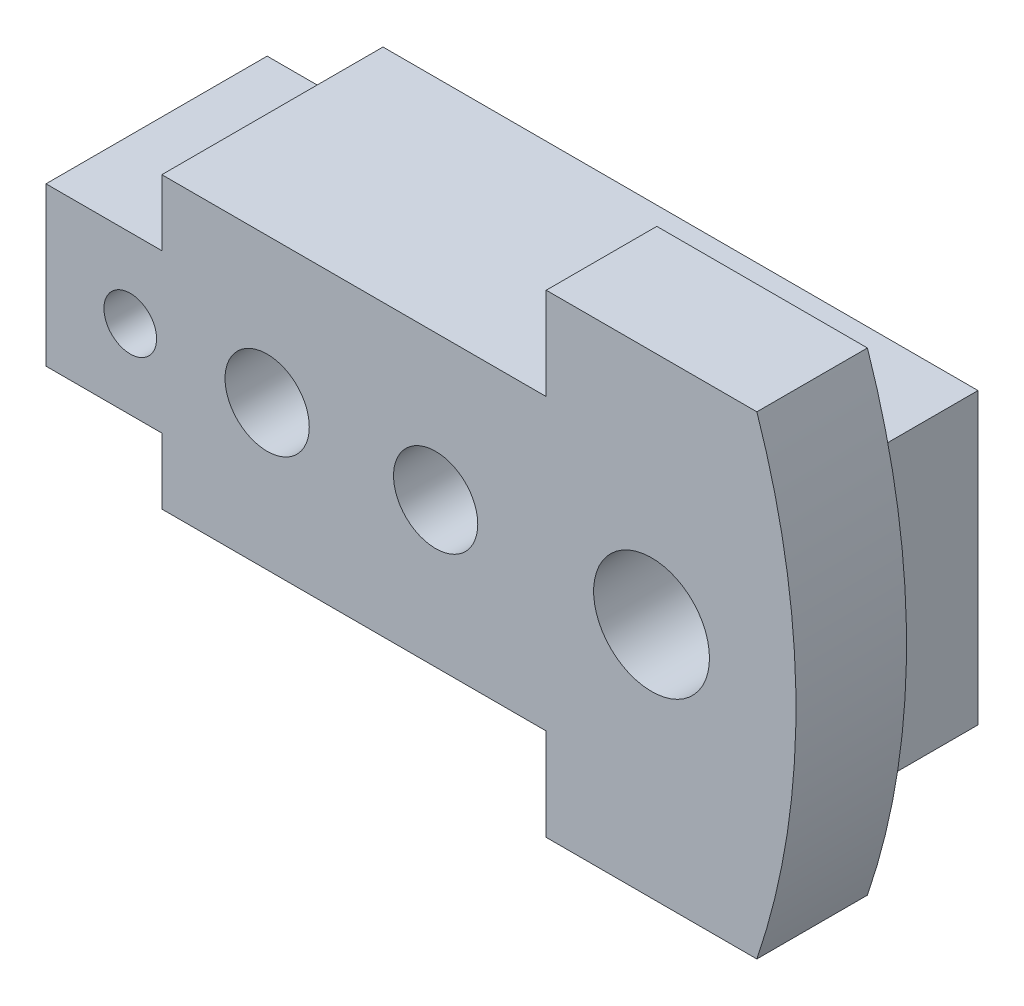
ISO-10303-21;
HEADER;
FILE_DESCRIPTION(('STEP AP214'),'2;1');
FILE_NAME('part.step','',(''),(''),'','','');
FILE_SCHEMA(('AUTOMOTIVE_DESIGN { 1 0 10303 214 1 1 1 1 }'));
ENDSEC;
DATA;
#1=APPLICATION_CONTEXT('core data for automotive mechanical design processes');
#2=APPLICATION_PROTOCOL_DEFINITION('international standard','automotive_design',2000,#1);
#3=PRODUCT_CONTEXT('',#1,'mechanical');
#4=PRODUCT('Part','Part','',(#3));
#5=PRODUCT_RELATED_PRODUCT_CATEGORY('part','',(#4));
#6=PRODUCT_DEFINITION_FORMATION('','',#4);
#7=PRODUCT_DEFINITION_CONTEXT('part definition',#1,'design');
#8=PRODUCT_DEFINITION('design','',#6,#7);
#9=PRODUCT_DEFINITION_SHAPE('','',#8);
#10=(LENGTH_UNIT() NAMED_UNIT(*) SI_UNIT(.MILLI.,.METRE.));
#11=(NAMED_UNIT(*) PLANE_ANGLE_UNIT() SI_UNIT($,.RADIAN.));
#12=(NAMED_UNIT(*) SI_UNIT($,.STERADIAN.) SOLID_ANGLE_UNIT());
#13=UNCERTAINTY_MEASURE_WITH_UNIT(LENGTH_MEASURE(1.E-05),#10,'distance_accuracy_value','');
#14=(GEOMETRIC_REPRESENTATION_CONTEXT(3) GLOBAL_UNCERTAINTY_ASSIGNED_CONTEXT((#13)) GLOBAL_UNIT_ASSIGNED_CONTEXT((#10,
#11,#12)) REPRESENTATION_CONTEXT('',''));
#15=CARTESIAN_POINT('',(0.,0.,0.));
#16=DIRECTION('',(0.,0.,1.));
#17=DIRECTION('',(1.,0.,0.));
#18=AXIS2_PLACEMENT_3D('',#15,#16,#17);
#19=CARTESIAN_POINT('',(0.,0.,0.));
#20=DIRECTION('',(0.,0.,1.));
#21=DIRECTION('',(1.,0.,0.));
#22=AXIS2_PLACEMENT_3D('',#19,#20,#21);
#23=PLANE('',#22);
#24=DIRECTION('',(0.,-1.,0.));
#25=VECTOR('',#24,1.);
#26=CARTESIAN_POINT('',(18.,0.,0.));
#27=LINE('',#26,#25);
#28=CARTESIAN_POINT('',(18.,72.5,0.));
#29=VERTEX_POINT('',#28);
#30=CARTESIAN_POINT('',(18.,60.,0.));
#31=VERTEX_POINT('',#30);
#32=EDGE_CURVE('E70',#29,#31,#27,.T.);
#33=ORIENTED_EDGE('',*,*,#32,.F.);
#34=DIRECTION('',(1.,0.,0.));
#35=VECTOR('',#34,1.);
#36=CARTESIAN_POINT('',(91.,72.5,0.));
#37=LINE('',#36,#35);
#38=CARTESIAN_POINT('',(131.,72.5,0.));
#39=VERTEX_POINT('',#38);
#40=EDGE_CURVE('E153',#29,#39,#37,.T.);
#41=ORIENTED_EDGE('',*,*,#40,.T.);
#42=DIRECTION('',(0.,1.,0.));
#43=VECTOR('',#42,1.);
#44=CARTESIAN_POINT('',(131.,90.,0.));
#45=LINE('',#44,#43);
#46=CARTESIAN_POINT('',(131.,17.5,0.));
#47=VERTEX_POINT('',#46);
#48=EDGE_CURVE('E188',#47,#39,#45,.T.);
#49=ORIENTED_EDGE('',*,*,#48,.F.);
#50=DIRECTION('',(1.,0.,0.));
#51=VECTOR('',#50,1.);
#52=CARTESIAN_POINT('',(91.,17.5,0.));
#53=LINE('',#52,#51);
#54=CARTESIAN_POINT('',(18.,17.5,0.));
#55=VERTEX_POINT('',#54);
#56=EDGE_CURVE('E234',#55,#47,#53,.T.);
#57=ORIENTED_EDGE('',*,*,#56,.F.);
#58=DIRECTION('',(0.,-1.,0.));
#59=VECTOR('',#58,1.);
#60=CARTESIAN_POINT('',(18.,0.,0.));
#61=LINE('',#60,#59);
#62=CARTESIAN_POINT('',(18.,30.,0.));
#63=VERTEX_POINT('',#62);
#64=EDGE_CURVE('E195',#63,#55,#61,.T.);
#65=ORIENTED_EDGE('',*,*,#64,.F.);
#66=DIRECTION('',(-1.,0.,0.));
#67=VECTOR('',#66,1.);
#68=CARTESIAN_POINT('',(0.,30.,0.));
#69=LINE('',#68,#67);
#70=CARTESIAN_POINT('',(-3.99999999999999,30.,0.));
#71=VERTEX_POINT('',#70);
#72=EDGE_CURVE('E204',#63,#71,#69,.T.);
#73=ORIENTED_EDGE('',*,*,#72,.T.);
#74=DIRECTION('',(0.,-1.,0.));
#75=VECTOR('',#74,1.);
#76=CARTESIAN_POINT('',(-3.99999999999999,90.,0.));
#77=LINE('',#76,#75);
#78=CARTESIAN_POINT('',(-3.99999999999999,60.,0.));
#79=VERTEX_POINT('',#78);
#80=EDGE_CURVE('E11',#79,#71,#77,.T.);
#81=ORIENTED_EDGE('',*,*,#80,.F.);
#82=DIRECTION('',(1.,0.,0.));
#83=VECTOR('',#82,1.);
#84=CARTESIAN_POINT('',(0.,60.,0.));
#85=LINE('',#84,#83);
#86=EDGE_CURVE('E192',#79,#31,#85,.T.);
#87=ORIENTED_EDGE('',*,*,#86,.T.);
#88=EDGE_LOOP('',(#33,#41,#49,#57,#65,#73,#81,#87));
#89=FACE_BOUND('',#88,.T.);
#90=ADVANCED_FACE('F44',(#89),#23,.F.);
#91=CARTESIAN_POINT('',(131.,0.,0.));
#92=DIRECTION('',(-1.,0.,0.));
#93=DIRECTION('',(0.,0.,1.));
#94=AXIS2_PLACEMENT_3D('',#91,#92,#93);
#95=PLANE('',#94);
#96=DIRECTION('',(0.,0.,1.));
#97=VECTOR('',#96,1.);
#98=CARTESIAN_POINT('',(131.,72.5,0.));
#99=LINE('',#98,#97);
#100=CARTESIAN_POINT('',(131.,72.5,21.));
#101=VERTEX_POINT('',#100);
#102=EDGE_CURVE('E232',#39,#101,#99,.T.);
#103=ORIENTED_EDGE('',*,*,#102,.T.);
#104=DIRECTION('',(0.,-1.,0.));
#105=VECTOR('',#104,1.);
#106=CARTESIAN_POINT('',(131.,90.,21.));
#107=LINE('',#106,#105);
#108=CARTESIAN_POINT('',(131.,17.5,21.));
#109=VERTEX_POINT('',#108);
#110=EDGE_CURVE('E173',#101,#109,#107,.T.);
#111=ORIENTED_EDGE('',*,*,#110,.T.);
#112=DIRECTION('',(0.,0.,-1.));
#113=VECTOR('',#112,1.);
#114=CARTESIAN_POINT('',(131.,17.5,0.));
#115=LINE('',#114,#113);
#116=EDGE_CURVE('E58',#109,#47,#115,.T.);
#117=ORIENTED_EDGE('',*,*,#116,.T.);
#118=ORIENTED_EDGE('',*,*,#48,.T.);
#119=EDGE_LOOP('',(#103,#111,#117,#118));
#120=FACE_BOUND('',#119,.T.);
#121=ADVANCED_FACE('F338',(#120),#95,.F.);
#122=CARTESIAN_POINT('',(0.,0.,63.));
#123=DIRECTION('',(0.,1.,0.));
#124=DIRECTION('',(0.,0.,1.));
#125=AXIS2_PLACEMENT_3D('',#122,#123,#124);
#126=PLANE('',#125);
#127=DIRECTION('',(1.,0.,0.));
#128=VECTOR('',#127,1.);
#129=CARTESIAN_POINT('',(91.,0.,42.));
#130=LINE('',#129,#128);
#131=CARTESIAN_POINT('',(91.,0.,42.));
#132=VERTEX_POINT('',#131);
#133=CARTESIAN_POINT('',(131.,0.,42.));
#134=VERTEX_POINT('',#133);
#135=EDGE_CURVE('E182',#132,#134,#130,.T.);
#136=ORIENTED_EDGE('',*,*,#135,.F.);
#137=DIRECTION('',(0.,0.,1.));
#138=VECTOR('',#137,1.);
#139=CARTESIAN_POINT('',(91.,0.,42.));
#140=LINE('',#139,#138);
#141=CARTESIAN_POINT('',(91.,0.,21.));
#142=VERTEX_POINT('',#141);
#143=EDGE_CURVE('E239',#142,#132,#140,.T.);
#144=ORIENTED_EDGE('',*,*,#143,.F.);
#145=DIRECTION('',(1.,0.,0.));
#146=VECTOR('',#145,1.);
#147=CARTESIAN_POINT('',(91.,0.,21.));
#148=LINE('',#147,#146);
#149=CARTESIAN_POINT('',(131.,0.,21.));
#150=VERTEX_POINT('',#149);
#151=EDGE_CURVE('E236',#142,#150,#148,.T.);
#152=ORIENTED_EDGE('',*,*,#151,.T.);
#153=DIRECTION('',(0.,0.,-1.));
#154=VECTOR('',#153,1.);
#155=CARTESIAN_POINT('',(131.,0.,0.));
#156=LINE('',#155,#154);
#157=EDGE_CURVE('E190',#134,#150,#156,.T.);
#158=ORIENTED_EDGE('',*,*,#157,.F.);
#159=EDGE_LOOP('',(#136,#144,#152,#158));
#160=FACE_BOUND('',#159,.T.);
#161=ADVANCED_FACE('F50',(#160),#126,.F.);
#162=CARTESIAN_POINT('',(22.,90.,63.));
#163=DIRECTION('',(0.,-1.,0.));
#164=DIRECTION('',(0.,0.,-1.));
#165=AXIS2_PLACEMENT_3D('',#162,#163,#164);
#166=PLANE('',#165);
#167=DIRECTION('',(1.,0.,0.));
#168=VECTOR('',#167,1.);
#169=CARTESIAN_POINT('',(91.,90.,21.));
#170=LINE('',#169,#168);
#171=CARTESIAN_POINT('',(91.,90.,21.));
#172=VERTEX_POINT('',#171);
#173=CARTESIAN_POINT('',(131.,90.,21.));
#174=VERTEX_POINT('',#173);
#175=EDGE_CURVE('E260',#172,#174,#170,.T.);
#176=ORIENTED_EDGE('',*,*,#175,.F.);
#177=DIRECTION('',(0.,0.,-1.));
#178=VECTOR('',#177,1.);
#179=CARTESIAN_POINT('',(91.,90.,0.));
#180=LINE('',#179,#178);
#181=CARTESIAN_POINT('',(91.,90.,42.));
#182=VERTEX_POINT('',#181);
#183=EDGE_CURVE('E156',#182,#172,#180,.T.);
#184=ORIENTED_EDGE('',*,*,#183,.F.);
#185=DIRECTION('',(-1.,0.,0.));
#186=VECTOR('',#185,1.);
#187=CARTESIAN_POINT('',(91.,90.,42.));
#188=LINE('',#187,#186);
#189=CARTESIAN_POINT('',(131.,90.,42.));
#190=VERTEX_POINT('',#189);
#191=EDGE_CURVE('E184',#190,#182,#188,.T.);
#192=ORIENTED_EDGE('',*,*,#191,.F.);
#193=DIRECTION('',(0.,0.,1.));
#194=VECTOR('',#193,1.);
#195=CARTESIAN_POINT('',(131.,90.,21.));
#196=LINE('',#195,#194);
#197=EDGE_CURVE('E166',#174,#190,#196,.T.);
#198=ORIENTED_EDGE('',*,*,#197,.F.);
#199=EDGE_LOOP('',(#176,#184,#192,#198));
#200=FACE_BOUND('',#199,.T.);
#201=ADVANCED_FACE('F281',(#200),#166,.F.);
#202=CARTESIAN_POINT('',(-3.99999999999999,90.,63.));
#203=DIRECTION('',(1.,0.,0.));
#204=DIRECTION('',(0.,0.,-1.));
#205=AXIS2_PLACEMENT_3D('',#202,#203,#204);
#206=PLANE('',#205);
#207=DIRECTION('',(0.,0.,1.));
#208=VECTOR('',#207,1.);
#209=CARTESIAN_POINT('',(-3.99999999999999,30.,0.));
#210=LINE('',#209,#208);
#211=CARTESIAN_POINT('',(-3.99999999999999,30.,42.));
#212=VERTEX_POINT('',#211);
#213=EDGE_CURVE('E199',#71,#212,#210,.T.);
#214=ORIENTED_EDGE('',*,*,#213,.T.);
#215=DIRECTION('',(0.,-1.,0.));
#216=VECTOR('',#215,1.);
#217=CARTESIAN_POINT('',(-3.99999999999999,30.,42.));
#218=LINE('',#217,#216);
#219=CARTESIAN_POINT('',(-3.99999999999999,60.,42.));
#220=VERTEX_POINT('',#219);
#221=EDGE_CURVE('E167',#220,#212,#218,.T.);
#222=ORIENTED_EDGE('',*,*,#221,.F.);
#223=DIRECTION('',(0.,0.,1.));
#224=VECTOR('',#223,1.);
#225=CARTESIAN_POINT('',(-3.99999999999999,60.,0.));
#226=LINE('',#225,#224);
#227=EDGE_CURVE('E198',#79,#220,#226,.T.);
#228=ORIENTED_EDGE('',*,*,#227,.F.);
#229=ORIENTED_EDGE('',*,*,#80,.T.);
#230=EDGE_LOOP('',(#214,#222,#228,#229));
#231=FACE_BOUND('',#230,.T.);
#232=ADVANCED_FACE('F226',(#231),#206,.F.);
#233=CARTESIAN_POINT('',(18.,0.,0.));
#234=DIRECTION('',(-1.,0.,0.));
#235=DIRECTION('',(0.,0.,1.));
#236=AXIS2_PLACEMENT_3D('',#233,#234,#235);
#237=PLANE('',#236);
#238=DIRECTION('',(0.,0.,-1.));
#239=VECTOR('',#238,1.);
#240=CARTESIAN_POINT('',(18.,17.5,0.));
#241=LINE('',#240,#239);
#242=CARTESIAN_POINT('',(18.,17.5,42.));
#243=VERTEX_POINT('',#242);
#244=EDGE_CURVE('E221',#243,#55,#241,.T.);
#245=ORIENTED_EDGE('',*,*,#244,.F.);
#246=DIRECTION('',(0.,-1.,0.));
#247=VECTOR('',#246,1.);
#248=CARTESIAN_POINT('',(18.,0.,42.));
#249=LINE('',#248,#247);
#250=CARTESIAN_POINT('',(18.,30.,42.));
#251=VERTEX_POINT('',#250);
#252=EDGE_CURVE('E179',#251,#243,#249,.T.);
#253=ORIENTED_EDGE('',*,*,#252,.F.);
#254=DIRECTION('',(0.,0.,1.));
#255=VECTOR('',#254,1.);
#256=CARTESIAN_POINT('',(18.,30.,0.));
#257=LINE('',#256,#255);
#258=EDGE_CURVE('E206',#63,#251,#257,.T.);
#259=ORIENTED_EDGE('',*,*,#258,.F.);
#260=ORIENTED_EDGE('',*,*,#64,.T.);
#261=EDGE_LOOP('',(#245,#253,#259,#260));
#262=FACE_BOUND('',#261,.T.);
#263=ADVANCED_FACE('F218',(#262),#237,.T.);
#264=CARTESIAN_POINT('',(0.,30.,0.));
#265=DIRECTION('',(0.,1.,0.));
#266=DIRECTION('',(-1.,0.,0.));
#267=AXIS2_PLACEMENT_3D('',#264,#265,#266);
#268=PLANE('',#267);
#269=ORIENTED_EDGE('',*,*,#258,.T.);
#270=DIRECTION('',(1.,0.,0.));
#271=VECTOR('',#270,1.);
#272=CARTESIAN_POINT('',(18.,30.,42.));
#273=LINE('',#272,#271);
#274=EDGE_CURVE('E178',#212,#251,#273,.T.);
#275=ORIENTED_EDGE('',*,*,#274,.F.);
#276=ORIENTED_EDGE('',*,*,#213,.F.);
#277=ORIENTED_EDGE('',*,*,#72,.F.);
#278=EDGE_LOOP('',(#269,#275,#276,#277));
#279=FACE_BOUND('',#278,.T.);
#280=ADVANCED_FACE('F213',(#279),#268,.F.);
#281=CARTESIAN_POINT('',(18.,0.,0.));
#282=DIRECTION('',(-1.,0.,0.));
#283=DIRECTION('',(0.,0.,1.));
#284=AXIS2_PLACEMENT_3D('',#281,#282,#283);
#285=PLANE('',#284);
#286=DIRECTION('',(0.,0.,1.));
#287=VECTOR('',#286,1.);
#288=CARTESIAN_POINT('',(18.,72.5,42.));
#289=LINE('',#288,#287);
#290=CARTESIAN_POINT('',(18.,72.5,42.));
#291=VERTEX_POINT('',#290);
#292=EDGE_CURVE('E150',#29,#291,#289,.T.);
#293=ORIENTED_EDGE('',*,*,#292,.F.);
#294=ORIENTED_EDGE('',*,*,#32,.T.);
#295=DIRECTION('',(0.,0.,1.));
#296=VECTOR('',#295,1.);
#297=CARTESIAN_POINT('',(18.,60.,0.));
#298=LINE('',#297,#296);
#299=CARTESIAN_POINT('',(18.,60.,42.));
#300=VERTEX_POINT('',#299);
#301=EDGE_CURVE('E52',#31,#300,#298,.T.);
#302=ORIENTED_EDGE('',*,*,#301,.T.);
#303=DIRECTION('',(0.,-1.,0.));
#304=VECTOR('',#303,1.);
#305=CARTESIAN_POINT('',(18.,60.,42.));
#306=LINE('',#305,#304);
#307=EDGE_CURVE('E163',#291,#300,#306,.T.);
#308=ORIENTED_EDGE('',*,*,#307,.F.);
#309=EDGE_LOOP('',(#293,#294,#302,#308));
#310=FACE_BOUND('',#309,.T.);
#311=ADVANCED_FACE('F168',(#310),#285,.T.);
#312=CARTESIAN_POINT('',(0.,60.,0.));
#313=DIRECTION('',(0.,-1.,0.));
#314=DIRECTION('',(0.,0.,-1.));
#315=AXIS2_PLACEMENT_3D('',#312,#313,#314);
#316=PLANE('',#315);
#317=ORIENTED_EDGE('',*,*,#227,.T.);
#318=DIRECTION('',(-1.,0.,0.));
#319=VECTOR('',#318,1.);
#320=CARTESIAN_POINT('',(-3.99999999999999,60.,42.));
#321=LINE('',#320,#319);
#322=EDGE_CURVE('E170',#300,#220,#321,.T.);
#323=ORIENTED_EDGE('',*,*,#322,.F.);
#324=ORIENTED_EDGE('',*,*,#301,.F.);
#325=ORIENTED_EDGE('',*,*,#86,.F.);
#326=EDGE_LOOP('',(#317,#323,#324,#325));
#327=FACE_BOUND('',#326,.T.);
#328=ADVANCED_FACE('F233',(#327),#316,.F.);
#329=CARTESIAN_POINT('',(0.,0.,42.));
#330=DIRECTION('',(0.,0.,-1.));
#331=DIRECTION('',(-1.,0.,0.));
#332=AXIS2_PLACEMENT_3D('',#329,#330,#331);
#333=PLANE('',#332);
#334=CARTESIAN_POINT('',(111.,45.,42.));
#335=DIRECTION('',(0.,0.,1.));
#336=DIRECTION('',(1.,0.,0.));
#337=AXIS2_PLACEMENT_3D('',#334,#335,#336);
#338=CIRCLE('',#337,11.);
#339=CARTESIAN_POINT('',(122.,45.,42.));
#340=VERTEX_POINT('',#339);
#341=EDGE_CURVE('E290',#340,#340,#338,.T.);
#342=ORIENTED_EDGE('',*,*,#341,.F.);
#343=EDGE_LOOP('',(#342));
#344=FACE_BOUND('',#343,.T.);
#345=CARTESIAN_POINT('',(70.,45.,42.));
#346=DIRECTION('',(0.,0.,1.));
#347=DIRECTION('',(1.,0.,0.));
#348=AXIS2_PLACEMENT_3D('',#345,#346,#347);
#349=CIRCLE('',#348,8.);
#350=CARTESIAN_POINT('',(78.,45.,42.));
#351=VERTEX_POINT('',#350);
#352=EDGE_CURVE('E303',#351,#351,#349,.T.);
#353=ORIENTED_EDGE('',*,*,#352,.F.);
#354=EDGE_LOOP('',(#353));
#355=FACE_BOUND('',#354,.T.);
#356=CARTESIAN_POINT('',(38.,45.,42.));
#357=DIRECTION('',(0.,0.,1.));
#358=DIRECTION('',(1.,0.,0.));
#359=AXIS2_PLACEMENT_3D('',#356,#357,#358);
#360=CIRCLE('',#359,8.);
#361=CARTESIAN_POINT('',(46.,45.,42.));
#362=VERTEX_POINT('',#361);
#363=EDGE_CURVE('E300',#362,#362,#360,.T.);
#364=ORIENTED_EDGE('',*,*,#363,.F.);
#365=EDGE_LOOP('',(#364));
#366=FACE_BOUND('',#365,.T.);
#367=CARTESIAN_POINT('',(12.,45.,42.));
#368=DIRECTION('',(0.,0.,1.));
#369=DIRECTION('',(1.,0.,0.));
#370=AXIS2_PLACEMENT_3D('',#367,#368,#369);
#371=CIRCLE('',#370,5.00000000000001);
#372=CARTESIAN_POINT('',(17.,45.,42.));
#373=VERTEX_POINT('',#372);
#374=EDGE_CURVE('E293',#373,#373,#371,.T.);
#375=ORIENTED_EDGE('',*,*,#374,.F.);
#376=EDGE_LOOP('',(#375));
#377=FACE_BOUND('',#376,.T.);
#378=ORIENTED_EDGE('',*,*,#191,.T.);
#379=DIRECTION('',(0.,1.,0.));
#380=VECTOR('',#379,1.);
#381=CARTESIAN_POINT('',(91.,72.5,42.));
#382=LINE('',#381,#380);
#383=CARTESIAN_POINT('',(91.,72.5,42.));
#384=VERTEX_POINT('',#383);
#385=EDGE_CURVE('E161',#384,#182,#382,.T.);
#386=ORIENTED_EDGE('',*,*,#385,.F.);
#387=DIRECTION('',(1.,0.,0.));
#388=VECTOR('',#387,1.);
#389=CARTESIAN_POINT('',(91.,72.5,42.));
#390=LINE('',#389,#388);
#391=EDGE_CURVE('E154',#291,#384,#390,.T.);
#392=ORIENTED_EDGE('',*,*,#391,.F.);
#393=ORIENTED_EDGE('',*,*,#307,.T.);
#394=ORIENTED_EDGE('',*,*,#322,.T.);
#395=ORIENTED_EDGE('',*,*,#221,.T.);
#396=ORIENTED_EDGE('',*,*,#274,.T.);
#397=ORIENTED_EDGE('',*,*,#252,.T.);
#398=DIRECTION('',(-1.,0.,0.));
#399=VECTOR('',#398,1.);
#400=CARTESIAN_POINT('',(18.,17.5,42.));
#401=LINE('',#400,#399);
#402=CARTESIAN_POINT('',(91.,17.5,42.));
#403=VERTEX_POINT('',#402);
#404=EDGE_CURVE('E222',#403,#243,#401,.T.);
#405=ORIENTED_EDGE('',*,*,#404,.F.);
#406=DIRECTION('',(0.,-1.,0.));
#407=VECTOR('',#406,1.);
#408=CARTESIAN_POINT('',(91.,17.5,42.));
#409=LINE('',#408,#407);
#410=EDGE_CURVE('E250',#403,#132,#409,.T.);
#411=ORIENTED_EDGE('',*,*,#410,.T.);
#412=ORIENTED_EDGE('',*,*,#135,.T.);
#413=CARTESIAN_POINT('',(-1.57073583562853,45.,42.));
#414=DIRECTION('',(0.,0.,1.));
#415=DIRECTION('',(-1.,0.,0.));
#416=AXIS2_PLACEMENT_3D('',#413,#414,#415);
#417=CIRCLE('',#416,140.);
#418=EDGE_CURVE('E256',#134,#190,#417,.T.);
#419=ORIENTED_EDGE('',*,*,#418,.T.);
#420=EDGE_LOOP('',(#378,#386,#392,#393,#394,#395,#396,#397,#405,#411,#412,#419));
#421=FACE_BOUND('',#420,.T.);
#422=ADVANCED_FACE('F159',(#344,#355,#366,#377,#421),#333,.F.);
#423=CARTESIAN_POINT('',(-1.57073583562853,45.,21.));
#424=DIRECTION('',(0.,0.,1.));
#425=DIRECTION('',(1.,0.,0.));
#426=AXIS2_PLACEMENT_3D('',#423,#424,#425);
#427=CYLINDRICAL_SURFACE('',#426,140.);
#428=ORIENTED_EDGE('',*,*,#418,.F.);
#429=ORIENTED_EDGE('',*,*,#157,.T.);
#430=CARTESIAN_POINT('',(-1.57073583562853,45.,21.));
#431=DIRECTION('',(0.,0.,1.));
#432=DIRECTION('',(-1.,0.,0.));
#433=AXIS2_PLACEMENT_3D('',#430,#431,#432);
#434=CIRCLE('',#433,140.);
#435=EDGE_CURVE('E270',#150,#174,#434,.T.);
#436=ORIENTED_EDGE('',*,*,#435,.T.);
#437=ORIENTED_EDGE('',*,*,#197,.T.);
#438=EDGE_LOOP('',(#428,#429,#436,#437));
#439=FACE_BOUND('',#438,.T.);
#440=ADVANCED_FACE('F276',(#439),#427,.T.);
#441=CARTESIAN_POINT('',(-1.57073583562853,45.,21.));
#442=DIRECTION('',(0.,0.,-1.));
#443=DIRECTION('',(-1.,0.,0.));
#444=AXIS2_PLACEMENT_3D('',#441,#442,#443);
#445=PLANE('',#444);
#446=ORIENTED_EDGE('',*,*,#435,.F.);
#447=ORIENTED_EDGE('',*,*,#151,.F.);
#448=DIRECTION('',(0.,-1.,0.));
#449=VECTOR('',#448,1.);
#450=CARTESIAN_POINT('',(91.,0.,21.));
#451=LINE('',#450,#449);
#452=CARTESIAN_POINT('',(91.,17.5,21.));
#453=VERTEX_POINT('',#452);
#454=EDGE_CURVE('E264',#453,#142,#451,.T.);
#455=ORIENTED_EDGE('',*,*,#454,.F.);
#456=DIRECTION('',(1.,0.,0.));
#457=VECTOR('',#456,1.);
#458=CARTESIAN_POINT('',(91.,17.5,21.));
#459=LINE('',#458,#457);
#460=EDGE_CURVE('E265',#453,#109,#459,.T.);
#461=ORIENTED_EDGE('',*,*,#460,.T.);
#462=ORIENTED_EDGE('',*,*,#110,.F.);
#463=DIRECTION('',(1.,0.,0.));
#464=VECTOR('',#463,1.);
#465=CARTESIAN_POINT('',(91.,72.5,21.));
#466=LINE('',#465,#464);
#467=CARTESIAN_POINT('',(91.,72.5,21.));
#468=VERTEX_POINT('',#467);
#469=EDGE_CURVE('E253',#468,#101,#466,.T.);
#470=ORIENTED_EDGE('',*,*,#469,.F.);
#471=DIRECTION('',(0.,-1.,0.));
#472=VECTOR('',#471,1.);
#473=CARTESIAN_POINT('',(91.,0.,21.));
#474=LINE('',#473,#472);
#475=EDGE_CURVE('E249',#172,#468,#474,.T.);
#476=ORIENTED_EDGE('',*,*,#475,.F.);
#477=ORIENTED_EDGE('',*,*,#175,.T.);
#478=EDGE_LOOP('',(#446,#447,#455,#461,#462,#470,#476,#477));
#479=FACE_BOUND('',#478,.T.);
#480=ADVANCED_FACE('F362',(#479),#445,.T.);
#481=CARTESIAN_POINT('',(91.,17.5,0.));
#482=DIRECTION('',(0.,-1.,0.));
#483=DIRECTION('',(0.,0.,-1.));
#484=AXIS2_PLACEMENT_3D('',#481,#482,#483);
#485=PLANE('',#484);
#486=ORIENTED_EDGE('',*,*,#116,.F.);
#487=ORIENTED_EDGE('',*,*,#460,.F.);
#488=DIRECTION('',(0.,0.,1.));
#489=VECTOR('',#488,1.);
#490=CARTESIAN_POINT('',(91.,17.5,42.));
#491=LINE('',#490,#489);
#492=EDGE_CURVE('E237',#453,#403,#491,.T.);
#493=ORIENTED_EDGE('',*,*,#492,.T.);
#494=ORIENTED_EDGE('',*,*,#404,.T.);
#495=ORIENTED_EDGE('',*,*,#244,.T.);
#496=ORIENTED_EDGE('',*,*,#56,.T.);
#497=EDGE_LOOP('',(#486,#487,#493,#494,#495,#496));
#498=FACE_BOUND('',#497,.T.);
#499=ADVANCED_FACE('F238',(#498),#485,.T.);
#500=CARTESIAN_POINT('',(91.,72.5,0.));
#501=DIRECTION('',(0.,1.,0.));
#502=DIRECTION('',(0.,0.,1.));
#503=AXIS2_PLACEMENT_3D('',#500,#501,#502);
#504=PLANE('',#503);
#505=ORIENTED_EDGE('',*,*,#102,.F.);
#506=ORIENTED_EDGE('',*,*,#40,.F.);
#507=ORIENTED_EDGE('',*,*,#292,.T.);
#508=ORIENTED_EDGE('',*,*,#391,.T.);
#509=DIRECTION('',(0.,0.,-1.));
#510=VECTOR('',#509,1.);
#511=CARTESIAN_POINT('',(91.,72.5,0.));
#512=LINE('',#511,#510);
#513=EDGE_CURVE('E165',#384,#468,#512,.T.);
#514=ORIENTED_EDGE('',*,*,#513,.T.);
#515=ORIENTED_EDGE('',*,*,#469,.T.);
#516=EDGE_LOOP('',(#505,#506,#507,#508,#514,#515));
#517=FACE_BOUND('',#516,.T.);
#518=ADVANCED_FACE('F147',(#517),#504,.T.);
#519=CARTESIAN_POINT('',(91.,17.5,42.));
#520=DIRECTION('',(1.,0.,0.));
#521=DIRECTION('',(0.,0.,-1.));
#522=AXIS2_PLACEMENT_3D('',#519,#520,#521);
#523=PLANE('',#522);
#524=ORIENTED_EDGE('',*,*,#454,.T.);
#525=ORIENTED_EDGE('',*,*,#143,.T.);
#526=ORIENTED_EDGE('',*,*,#410,.F.);
#527=ORIENTED_EDGE('',*,*,#492,.F.);
#528=EDGE_LOOP('',(#524,#525,#526,#527));
#529=FACE_BOUND('',#528,.T.);
#530=ADVANCED_FACE('F337',(#529),#523,.F.);
#531=CARTESIAN_POINT('',(91.,72.5,0.));
#532=DIRECTION('',(1.,0.,0.));
#533=DIRECTION('',(0.,0.,-1.));
#534=AXIS2_PLACEMENT_3D('',#531,#532,#533);
#535=PLANE('',#534);
#536=ORIENTED_EDGE('',*,*,#475,.T.);
#537=ORIENTED_EDGE('',*,*,#513,.F.);
#538=ORIENTED_EDGE('',*,*,#385,.T.);
#539=ORIENTED_EDGE('',*,*,#183,.T.);
#540=EDGE_LOOP('',(#536,#537,#538,#539));
#541=FACE_BOUND('',#540,.T.);
#542=ADVANCED_FACE('F329',(#541),#535,.F.);
#543=CARTESIAN_POINT('',(12.,45.,12.));
#544=DIRECTION('',(0.,0.,1.));
#545=DIRECTION('',(1.,0.,0.));
#546=AXIS2_PLACEMENT_3D('',#543,#544,#545);
#547=CYLINDRICAL_SURFACE('',#546,5.00000000000001);
#548=CARTESIAN_POINT('',(12.,45.,12.));
#549=DIRECTION('',(0.,0.,1.));
#550=DIRECTION('',(1.,0.,0.));
#551=AXIS2_PLACEMENT_3D('',#548,#549,#550);
#552=CIRCLE('',#551,5.00000000000001);
#553=CARTESIAN_POINT('',(17.,45.,12.));
#554=VERTEX_POINT('',#553);
#555=EDGE_CURVE('E295',#554,#554,#552,.T.);
#556=ORIENTED_EDGE('',*,*,#555,.F.);
#557=EDGE_LOOP('',(#556));
#558=FACE_BOUND('',#557,.T.);
#559=ORIENTED_EDGE('',*,*,#374,.T.);
#560=EDGE_LOOP('',(#559));
#561=FACE_BOUND('',#560,.T.);
#562=ADVANCED_FACE('F325',(#558,#561),#547,.F.);
#563=CARTESIAN_POINT('',(12.,45.,12.));
#564=DIRECTION('',(0.,0.,1.));
#565=DIRECTION('',(1.,0.,0.));
#566=AXIS2_PLACEMENT_3D('',#563,#564,#565);
#567=PLANE('',#566);
#568=ORIENTED_EDGE('',*,*,#555,.T.);
#569=EDGE_LOOP('',(#568));
#570=FACE_BOUND('',#569,.T.);
#571=ADVANCED_FACE('F322',(#570),#567,.T.);
#572=CARTESIAN_POINT('',(38.,45.,12.));
#573=DIRECTION('',(0.,0.,1.));
#574=DIRECTION('',(1.,0.,0.));
#575=AXIS2_PLACEMENT_3D('',#572,#573,#574);
#576=CYLINDRICAL_SURFACE('',#575,8.);
#577=CARTESIAN_POINT('',(38.,45.,12.));
#578=DIRECTION('',(0.,0.,1.));
#579=DIRECTION('',(1.,0.,0.));
#580=AXIS2_PLACEMENT_3D('',#577,#578,#579);
#581=CIRCLE('',#580,8.);
#582=CARTESIAN_POINT('',(46.,45.,12.));
#583=VERTEX_POINT('',#582);
#584=EDGE_CURVE('E297',#583,#583,#581,.T.);
#585=ORIENTED_EDGE('',*,*,#584,.F.);
#586=EDGE_LOOP('',(#585));
#587=FACE_BOUND('',#586,.T.);
#588=ORIENTED_EDGE('',*,*,#363,.T.);
#589=EDGE_LOOP('',(#588));
#590=FACE_BOUND('',#589,.T.);
#591=ADVANCED_FACE('F335',(#587,#590),#576,.F.);
#592=CARTESIAN_POINT('',(38.,45.,12.));
#593=DIRECTION('',(0.,0.,1.));
#594=DIRECTION('',(1.,0.,0.));
#595=AXIS2_PLACEMENT_3D('',#592,#593,#594);
#596=PLANE('',#595);
#597=ORIENTED_EDGE('',*,*,#584,.T.);
#598=EDGE_LOOP('',(#597));
#599=FACE_BOUND('',#598,.T.);
#600=ADVANCED_FACE('F445',(#599),#596,.T.);
#601=CARTESIAN_POINT('',(70.,45.,12.));
#602=DIRECTION('',(0.,0.,1.));
#603=DIRECTION('',(1.,0.,0.));
#604=AXIS2_PLACEMENT_3D('',#601,#602,#603);
#605=CYLINDRICAL_SURFACE('',#604,8.);
#606=CARTESIAN_POINT('',(70.,45.,12.));
#607=DIRECTION('',(0.,0.,1.));
#608=DIRECTION('',(1.,0.,0.));
#609=AXIS2_PLACEMENT_3D('',#606,#607,#608);
#610=CIRCLE('',#609,8.);
#611=CARTESIAN_POINT('',(78.,45.,12.));
#612=VERTEX_POINT('',#611);
#613=EDGE_CURVE('E306',#612,#612,#610,.T.);
#614=ORIENTED_EDGE('',*,*,#613,.F.);
#615=EDGE_LOOP('',(#614));
#616=FACE_BOUND('',#615,.T.);
#617=ORIENTED_EDGE('',*,*,#352,.T.);
#618=EDGE_LOOP('',(#617));
#619=FACE_BOUND('',#618,.T.);
#620=ADVANCED_FACE('F453',(#616,#619),#605,.F.);
#621=CARTESIAN_POINT('',(70.,45.,12.));
#622=DIRECTION('',(0.,0.,1.));
#623=DIRECTION('',(1.,0.,0.));
#624=AXIS2_PLACEMENT_3D('',#621,#622,#623);
#625=PLANE('',#624);
#626=ORIENTED_EDGE('',*,*,#613,.T.);
#627=EDGE_LOOP('',(#626));
#628=FACE_BOUND('',#627,.T.);
#629=ADVANCED_FACE('F467',(#628),#625,.T.);
#630=CARTESIAN_POINT('',(111.,45.,12.));
#631=DIRECTION('',(0.,0.,1.));
#632=DIRECTION('',(1.,0.,0.));
#633=AXIS2_PLACEMENT_3D('',#630,#631,#632);
#634=CYLINDRICAL_SURFACE('',#633,11.);
#635=CARTESIAN_POINT('',(111.,45.,12.));
#636=DIRECTION('',(0.,0.,1.));
#637=DIRECTION('',(1.,0.,0.));
#638=AXIS2_PLACEMENT_3D('',#635,#636,#637);
#639=CIRCLE('',#638,11.);
#640=CARTESIAN_POINT('',(122.,45.,12.));
#641=VERTEX_POINT('',#640);
#642=EDGE_CURVE('E282',#641,#641,#639,.T.);
#643=ORIENTED_EDGE('',*,*,#642,.F.);
#644=EDGE_LOOP('',(#643));
#645=FACE_BOUND('',#644,.T.);
#646=ORIENTED_EDGE('',*,*,#341,.T.);
#647=EDGE_LOOP('',(#646));
#648=FACE_BOUND('',#647,.T.);
#649=ADVANCED_FACE('F315',(#645,#648),#634,.F.);
#650=CARTESIAN_POINT('',(111.,45.,12.));
#651=DIRECTION('',(0.,0.,1.));
#652=DIRECTION('',(1.,0.,0.));
#653=AXIS2_PLACEMENT_3D('',#650,#651,#652);
#654=PLANE('',#653);
#655=ORIENTED_EDGE('',*,*,#642,.T.);
#656=EDGE_LOOP('',(#655));
#657=FACE_BOUND('',#656,.T.);
#658=ADVANCED_FACE('F490',(#657),#654,.T.);
#659=CLOSED_SHELL('',(#90,#121,#161,#201,#232,#263,#280,#311,#328,#422,#440,#480,#499,#518,#530,
#542,#562,#571,#591,#600,#620,#629,#649,#658));
#660=MANIFOLD_SOLID_BREP('B2',#659);
#661=ADVANCED_BREP_SHAPE_REPRESENTATION('',(#18,#660),#14);
#662=SHAPE_DEFINITION_REPRESENTATION(#9,#661);
ENDSEC;
END-ISO-10303-21;
